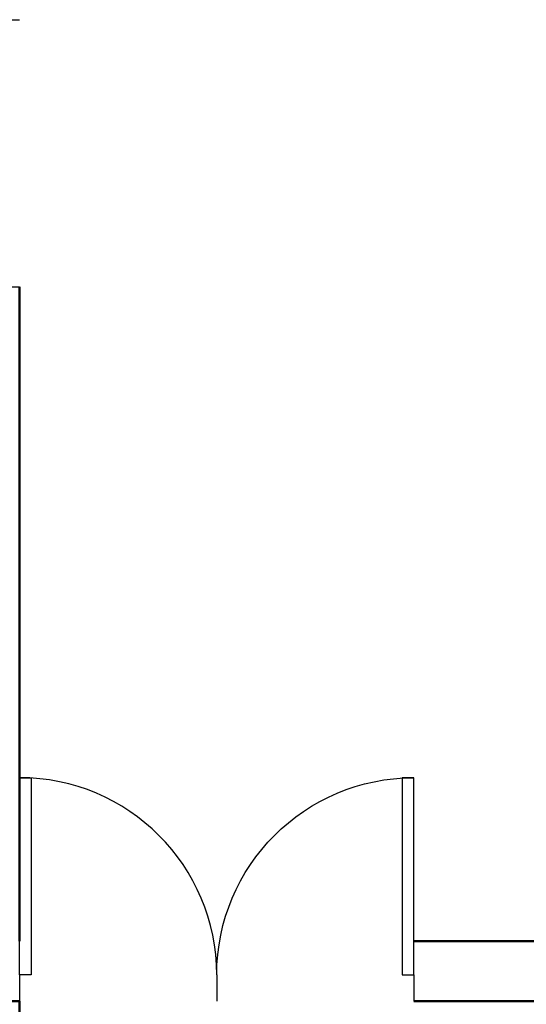
# Model space of a CAD drawing. Units: inches. Extents: x -105 to 1196, y -792 to 119.
# Tile 10 of 23: x 130 to 206, y -439 to -291. Entities that reach past the tile are written whole.
import ezdxf

# ---------------------------------------------------------------- set-up
doc = ezdxf.new("R2010")
doc.units = ezdxf.units.IN
doc.header["$MEASUREMENT"] = 0
doc.layers.add('A-DOOR', color=4, linetype='Continuous', lineweight=25)
doc.layers.add('A-WALL', color=3, linetype='Continuous', lineweight=50)

# ---------------------------------------------------------------- blocks, each defined once
blk = doc.blocks.new('*U17')
for p, q in [((0, 0), (0, -100)), ((750, 0), (750, -100))]:
    blk.add_line(p, q)
blk.add_lwpolyline([(0, 0), (0, 750), (43.75, 750), (43.75, 0)], close=True)
blk.add_arc((0, 0), 750, 0, 90)
blk = doc.blocks.new('*U25')
for p, q in [((0, 0), (0, -6)), ((-40, 0), (-40, -6))]:
    blk.add_line(p, q)
blk.add_lwpolyline([(0, 0), (0, 40), (-1.75, 40), (-1.75, 0)], close=True)
blk.add_arc((0, 0), 40, 90, 180)

msp = doc.modelspace()

# ---------------------------------------------------------------- linework, layer by layer
at = {"layer": 'A-WALL'}
for p, q in [((129.74, -429.23), (129.74, -331.23)), ((188.8, -429.23), (314.74, -429.23)), ((-45.26, -438.23), (129.74, -438.23)), ((129.74, -438.23), (129.74, -508.23)), ((188.8, -438.23), (323.74, -438.23))]:
    msp.add_line(p, q, dxfattribs=at)

# ---------------------------------------------------------------- block references
at = {"layer": 'A-DOOR', "rotation": 90}
msp.add_blockref('*U25', (123.74, -291.23), dxfattribs=at)
at = {"layer": 'A-DOOR', "yscale": 0.0393700787401575, "zscale": 0.0393700787401575}
for p, xscale in [((129.74, -434.29), 0.0393700787401575), ((188.8, -434.29), -0.0393700787401575)]:
    msp.add_blockref('*U17', p, dxfattribs=dict(at, xscale=xscale))

doc.saveas('drawing.dxf')
